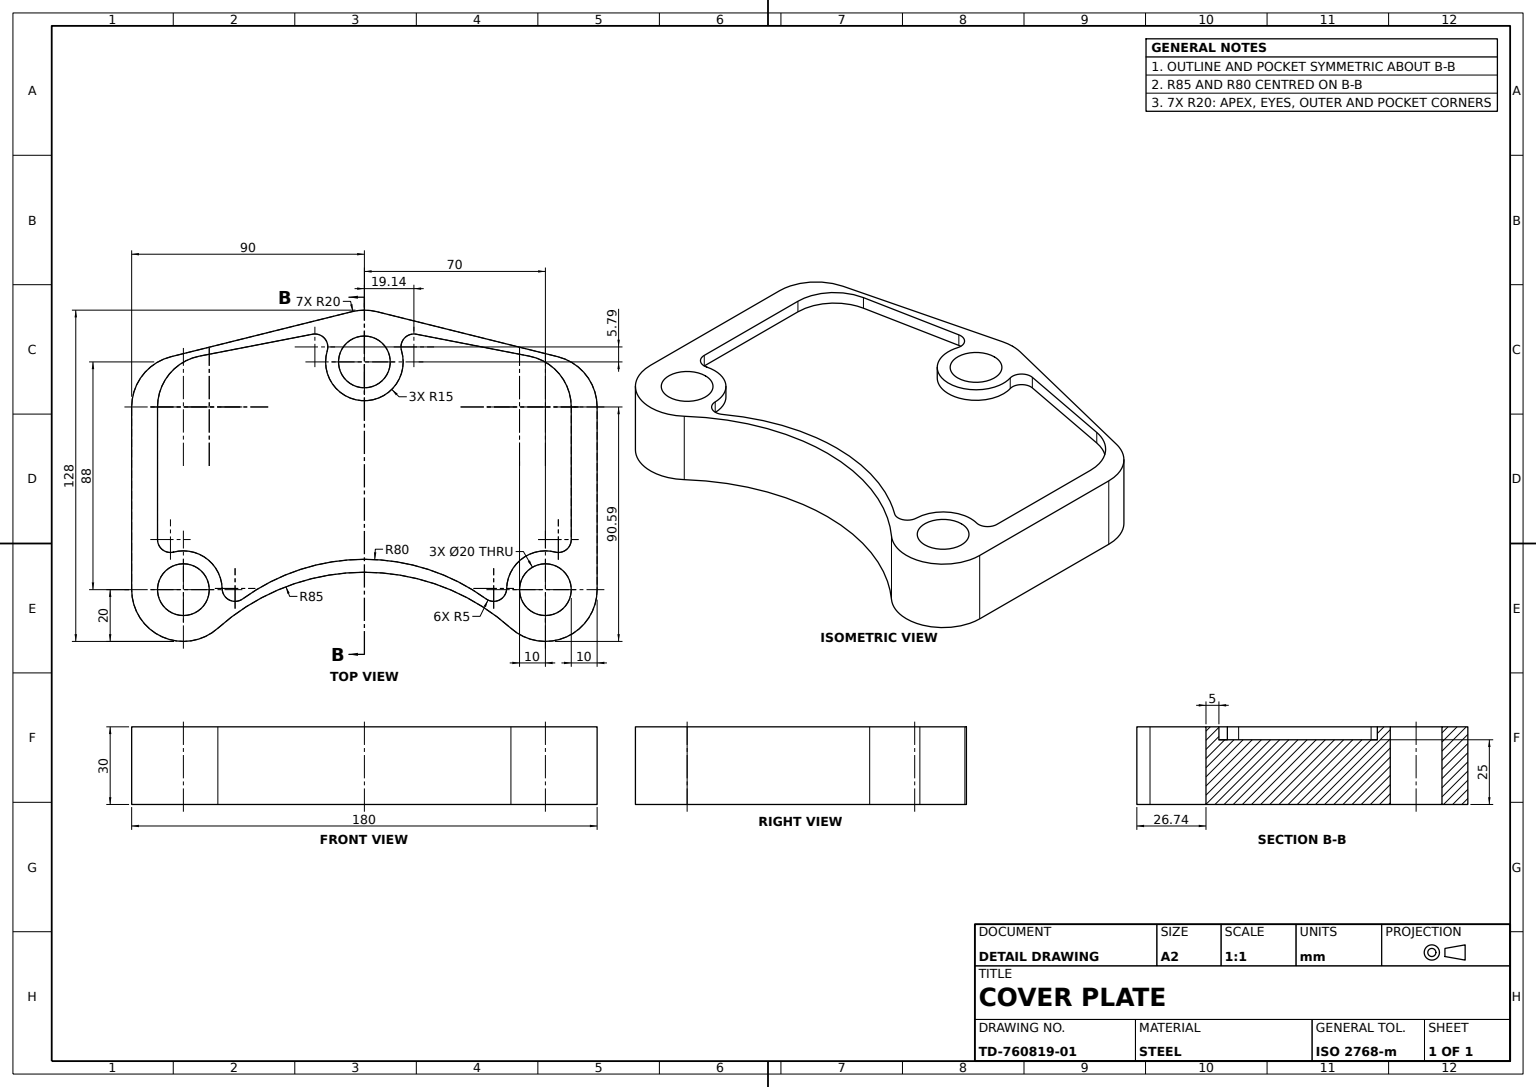
from build123d import *

# Parameters (mm, degrees)
PLATE_OUTLINE_SKETCH_R = 10
BASE_PLATE_30MM_DEPTH  = 30
TOP_POCKET_CUT_DEPTH   = 25


with BuildPart() as part:
    # Plate Outline Sketch → Base Plate 30mm (new body)
    with BuildSketch(Plane(origin=(0, 0, 0), x_dir=(1, 0, 0), z_dir=(0, 1, 0))):
        with BuildLine():
            Line((-90, -88), (-90, -17.408786158))
            ThreePointArc((-90, -17.408786158), (-85.756556041, -5.090874739), (-74.826905826, 2))
            Line((-74.826905826, 2), (-4.826905826, 19.408786158))
            ThreePointArc((-4.826905826, 19.408786158), (0, 20), (4.826905826, 19.408786158))
            Line((4.826905826, 19.408786158), (74.826905826, 2))
            ThreePointArc((74.826905826, 2), (85.756556041, -5.090874739), (90, -17.408786158))
            Line((90, -17.408786158), (90, -88))
            ThreePointArc((90, -88), (78.164965809, -106.257418584), (56.666666667, -102.90711985))
            ThreePointArc((56.666666667, -102.90711985), (0, -81.262379212), (-56.666666667, -102.90711985))
            ThreePointArc((-56.666666667, -102.90711985), (-78.164965809, -106.257418584), (-90, -88))
        make_face()
        with Locations(Location((0, 0, 0), (0, 0, 270))):
            Circle(PLATE_OUTLINE_SKETCH_R, mode=Mode.SUBTRACT)
        with Locations(Location((-70, -88, 0), (0, 0, 270))):
            Circle(PLATE_OUTLINE_SKETCH_R, mode=Mode.SUBTRACT)
        with Locations(Location((70, -88, 0), (0, 0, 90))):
            Circle(PLATE_OUTLINE_SKETCH_R, mode=Mode.SUBTRACT)
        with BuildLine():
            Line((-80, -68.635083269), (-80, -17.408786158))
            ThreePointArc((-80, -17.408786158), (-75.428711332, -4.682637227), (-63.804513336, 2.226021665))
            Line((-63.804513336, 2.226021665), (-20.095749168, 10.695194253))
            ThreePointArc((-20.095749168, 10.695194253), (-15.433233379, 9.136955423), (-14.358465626, 4.339869223))
            ThreePointArc((-14.358465626, 4.339869223), (0, -15), (14.358465626, 4.339869223))
            ThreePointArc((14.358465626, 4.339869223), (15.433233379, 9.136955423), (20.095749168, 10.695194253))
            Line((20.095749168, 10.695194253), (63.804513336, 2.226021665))
            ThreePointArc((63.804513336, 2.226021665), (75.428711332, -4.682637227), (80, -17.408786158))
            Line((80, -17.408786158), (80, -68.635083269))
            ThreePointArc((80, -68.635083269), (78.061862178, -72.587930344), (73.75, -73.476312452))
            ThreePointArc((73.75, -73.476312452), (60.955053625, -76.033841674), (55.004181334, -87.645849573))
            ThreePointArc((55.004181334, -87.645849573), (52.221345421, -92.010026772), (47.064070693, -91.571010006))
            ThreePointArc((47.064070693, -91.571010006), (0, -76.262379212), (-47.064070693, -91.571010006))
            ThreePointArc((-47.064070693, -91.571010006), (-52.221345421, -92.010026772), (-55.004181334, -87.645849573))
            ThreePointArc((-55.004181334, -87.645849573), (-60.955053625, -76.033841674), (-73.75, -73.476312452))
            ThreePointArc((-73.75, -73.476312452), (-78.061862178, -72.587930344), (-80, -68.635083269))
        make_face(mode=Mode.SUBTRACT)
    extrude(amount=BASE_PLATE_30MM_DEPTH)

    # Top Pocket Sketch → Top Pocket Cut (add)
    with BuildSketch(Plane.XZ):
        with BuildLine():
            Line((-20.095749168, -10.695194253), (-63.804513336, -2.226021665))
            ThreePointArc((-63.804513336, -2.226021665), (-75.428711332, 4.682637227), (-80, 17.408786158))
            Line((-80, 17.408786158), (-80, 68.635083269))
            ThreePointArc((-80, 68.635083269), (-78.061862178, 72.587930344), (-73.75, 73.476312452))
            ThreePointArc((-73.75, 73.476312452), (-60.955053625, 76.033841674), (-55.004181334, 87.645849573))
            ThreePointArc((-55.004181334, 87.645849573), (-52.221345421, 92.010026772), (-47.064070693, 91.571010006))
            ThreePointArc((-47.064070693, 91.571010006), (0, 76.262379212), (47.064070693, 91.571010006))
            ThreePointArc((47.064070693, 91.571010006), (52.221345421, 92.010026772), (55.004181334, 87.645849573))
            ThreePointArc((55.004181334, 87.645849573), (60.955053625, 76.033841674), (73.75, 73.476312452))
            ThreePointArc((73.75, 73.476312452), (78.061862178, 72.587930344), (80, 68.635083269))
            Line((80, 68.635083269), (80, 17.408786158))
            ThreePointArc((80, 17.408786158), (75.428711332, 4.682637227), (63.804513336, -2.226021665))
            Line((63.804513336, -2.226021665), (20.095749168, -10.695194253))
            ThreePointArc((20.095749168, -10.695194253), (15.433233379, -9.136955423), (14.358465626, -4.339869223))
            ThreePointArc((14.358465626, -4.339869223), (0, 15), (-14.358465626, -4.339869223))
            ThreePointArc((-14.358465626, -4.339869223), (-15.433233379, -9.136955423), (-20.095749168, -10.695194253))
        make_face()
    extrude(amount=-TOP_POCKET_CUT_DEPTH)


solid = part.part
